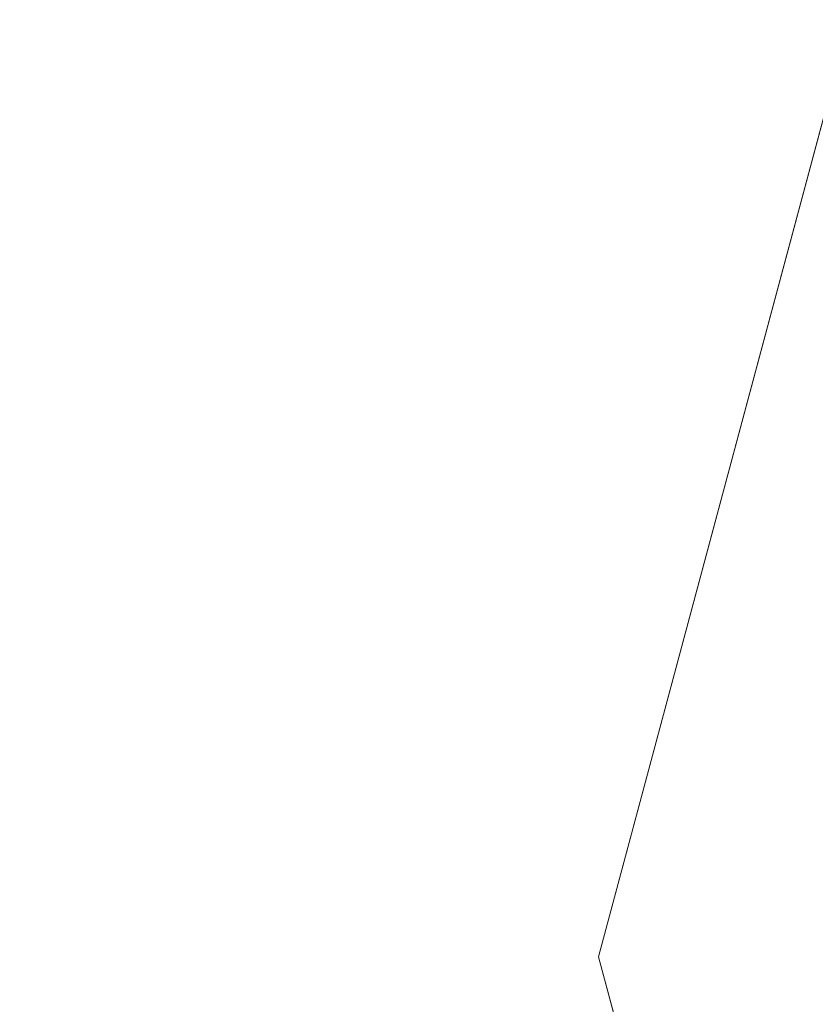
# Model space of a CAD drawing. Units: inches. Extents: x 375 to 1122, y 27 to 1069.
# Tile 29 of 155: x 732.625 to 734.833, y 277.109 to 279.842. Entities that reach past the tile are written whole.
import ezdxf

# ---------------------------------------------------------------- set-up
doc = ezdxf.new("R2010")
doc.units = ezdxf.units.IN
doc.layers.add('A-ANNO-DIMS', color=2, linetype='Continuous', lineweight=18)
doc.layers.add('Furniture', color=30, linetype='Continuous', lineweight=18)
doc.styles.get("Standard").update_dxf_attribs({"font": 'arial.ttf'})
doc.dimstyles.new('ISO-25', dxfattribs={"dimtxt": 12, "dimasz": 2.5, "dimexe": 1.5, "dimexo": 1.5, "dimtad": 1, "dimdec": 1, "dimlunit": 3, "dimtxsty": 'Standard', "dimblk": 'ARCHTICK', "dimcen": 2.5, "dimadec": 0, "dimazin": 0, "dimtfac": 1, "dimtdec": 1, "dimtmove": 0, "dimatfit": 3, "dimfxl": 1.5, "dimfxlon": 1, "dimarcsym": 0})

# ---------------------------------------------------------------- blocks, each defined once
blk = doc.blocks.new('A$C403C54AD')
at = {"linetype": 'ByBlock', "invisible_edges": 5}
for points in [[(1.674179, 1.280047, -0.037345), (1.657248, 1.250721, -0.02811), (1.726512, 1.232162, -0.02811), (1.726512, 1.266024, -0.037345)], [(1.726512, 1.266024, -0.037345), (1.726512, 1.232162, -0.02811), (1.795775, 1.250721, -0.02811), (1.778844, 1.280047, -0.037345)], [(1.657248, 1.250721, -0.023492), (1.666483, 1.266717, -0.023492), (1.726512, 1.250632, -0.023492), (1.726512, 1.232162, -0.023492)], [(1.726512, 1.232162, -0.023492), (1.726512, 1.250632, -0.023492), (1.78654, 1.266717, -0.023492), (1.795775, 1.250721, -0.023492)]]:
    blk.add_3dface(points, dxfattribs=at)
at = {"linetype": 'ByBlock'}
for points in [[(1.657248, 1.250721, -0.02811), (1.657248, 1.250721, -0.023492), (1.726512, 1.232162, -0.023492), (1.726512, 1.232162, -0.02811)], [(1.726512, 1.232162, -0.02811), (1.726512, 1.232162, -0.023492), (1.795775, 1.250721, -0.023492), (1.795775, 1.250721, -0.02811)]]:
    blk.add_3dface(points, dxfattribs=at)
blk = doc.blocks.new('_ArchTick')
at = {"color": 0, "linetype": 'ByBlock', "const_width": 0.15}
blk.add_lwpolyline([(-0.5, -0.5), (0.5, 0.5)], dxfattribs=at)
blk = doc.blocks.new('*D94')
at = {"layer": 'A-ANNO-DIMS', "color": 0, "lineweight": -2, "transparency": 16777216}
for p, q in [((734.0073, 117.5277), (734.0073, 114.5277)), ((773.0073, 117.5277), (773.0073, 114.5277)), ((734.0073, 116.0277), (773.0073, 116.0277))]:
    blk.add_line(p, q, dxfattribs=at)
at = {"layer": 'Defpoints', "color": 0, "transparency": 16777216}
for p in [(734.0073, 667.5277), (773.0073, 667.5277), (773.0073, 116.0277)]:
    blk.add_point(p, dxfattribs=at)
at = {"layer": 'A-ANNO-DIMS', "color": 0, "lineweight": -2, "transparency": 16777216, "xscale": 2.5, "yscale": 2.5, "zscale": 2.5, "rotation": 180}
blk.add_blockref('_ArchTick', (734.0073, 116.0277), dxfattribs=at)
at = {"layer": 'A-ANNO-DIMS', "color": 0, "lineweight": -2, "transparency": 16777216, "xscale": 2.5, "yscale": 2.5, "zscale": 2.5}
blk.add_blockref('_ArchTick', (773.0073, 116.0277), dxfattribs=at)
at = {"layer": 'A-ANNO-DIMS', "color": 0, "transparency": 16777216, "insert": (753.5073, 122.7837), "char_height": 12, "attachment_point": 5}
blk.add_mtext('3\'-3"', dxfattribs=at)

msp = doc.modelspace()

# ---------------------------------------------------------------- block references
at = {"layer": 'Furniture', "xscale": 39.9918517141215, "yscale": 39.9918517141215, "zscale": 39.9918517141215, "rotation": 270}
msp.add_blockref('A$C403C54AD', (684.9549, 346.2875, 0.024), dxfattribs=at)

# ---------------------------------------------------------------- dimensions: what is measured, and where the dimension line sits
at = {"layer": 'A-ANNO-DIMS'}
dim = msp.add_linear_dim(base=(773.0073, 116.0277), p1=(734.0073, 667.5277), p2=(773.0073, 667.5277), dimstyle='ISO-25', override={"dimdec": 1, "dimlfac": 1, "dimrnd": 0, "dimzin": 1, "dimdsep": 46, "dimlunit": 4, "dimfrac": 2}, dxfattribs=at)
dim.commit()
dim.dimension.update_dxf_attribs({"geometry": '*D94', "text_midpoint": (753.5073, 122.7837)})

doc.saveas('drawing.dxf')
